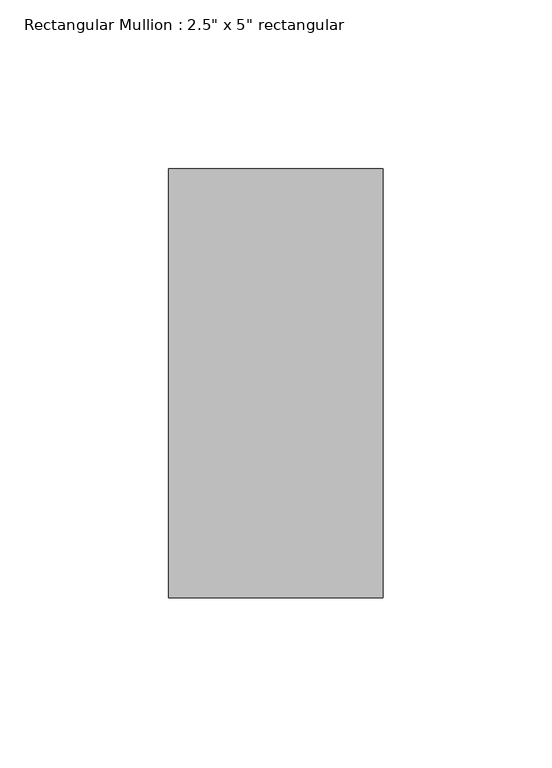
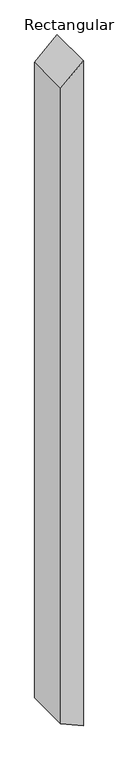
"""IFC4 building model written with IfcOpenShell, lengths in millimetres: member geometry."""

from ifc_helpers import new_model, si_unit, frame, origin, place, context, project, spatial, polyline, outline, extrude, source, transform, mapped, element, save


def member_129d910c(model_context):
    return source(origin(), model_context, "Body", "SweptSolid", [
        extrude(outline(polyline([(0.0, 0.0), (-59.214708, -63.5), (-1948.8698589, -63.5), (-1976.4804447, 0.0), (0.0, 0.0)])), frame((0.0, -63.5, 0.0), z_axis=(0.0, 1.0, 0.0), x_axis=(0.0, 0.0, 1.0)), (0.0, 0.0, 1.0), 127.0),
    ])


if __name__ == "__main__":
    model = new_model("IFC4")
    model_context = context("Model", 3, world=origin())
    ifc_project = project(units=[si_unit("LENGTHUNIT", "METRE", prefix="MILLI")], contexts=[model_context])
    site = spatial("IfcSite", under=ifc_project)
    building = spatial("IfcBuilding", under=site)
    placement = place(None, origin())
    member_shape = member_129d910c(model_context)
    element("IfcMember", 1, ObjectType="Rectangular Mullion : 2.5\" x 5\" rectangular", at=placement, inside=building, context=model_context, shape_type="MappedRepresentation", body=[
        mapped(member_shape, transform((0.0, 0.0, 0.0), x_axis=(1.0, 0.0, 0.0), y_axis=(0.0, 1.0, 0.0), z_axis=(0.0, 0.0, 1.0))),
    ])
    save(model, "model.ifc")

# Revit data of these elements
# Type "Rectangular Mullion : 2.5\" x 5\" rectangular"
#   built-in parameter 1007304 = 0.416667 (stored number, unit not read)
#   built-in parameter 1007301 = 0.104167 (stored number, unit not read)
#   built-in parameter 1007300 = 0.104167 (stored number, unit not read)
# Element 1 (IfcMember, "Rectangular Mullion : 2.5\" x 5\" rectangular")
#   Materials on its faces: "door colour"
# Materials
#   "door colour": class "Generic", colour RGB 120 120 120, transparency 0, Cost = 0
